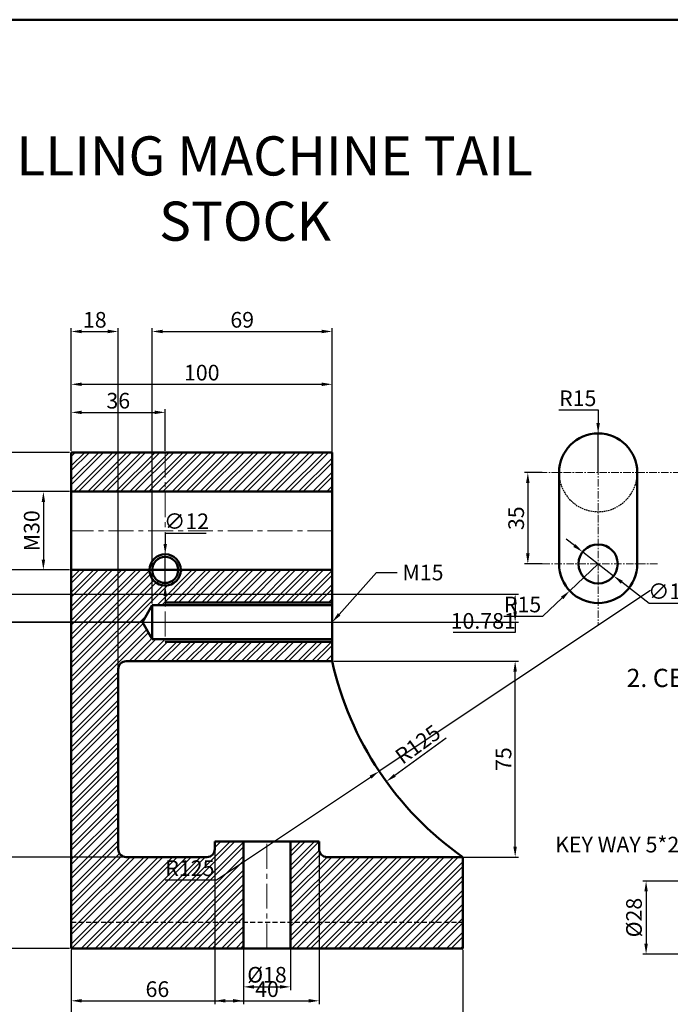
# Model space of a CAD drawing. Units: millimetres. Extents: x 177 to 1064, y 105 to 671.
# Tile 3 of 4: x 480 to 730, y 294 to 671. Entities that reach past the tile are written whole.
import ezdxf
from ezdxf import colors
from ezdxf.entities.mleader import LeaderData, LeaderLine
from ezdxf.math import Vec2, Vec3

# ---------------------------------------------------------------- set-up
doc = ezdxf.new("R2010")
doc.units = ezdxf.units.MM
doc.header["$LTSCALE"] = 0.3
doc.linetypes.add('CENTER', pattern=[50.8, 31.75, -6.35, 6.35, -6.35])
doc.linetypes.add('HIDDEN', pattern=[9.525, 6.35, -3.175])
for name, color, linetype, lineweight in [('M-CNTR', 1, 'CENTER', 18), ('M-DIMS', 2, 'Continuous', 25), ('M-HATC', 8, 'Continuous', 18), ('M-HIDN', 6, 'HIDDEN', 25), ('M-OUTL', 7, 'Continuous', 50), ('M-TEXT', 3, 'Continuous', 25)]:
    doc.layers.add(name, color=color, linetype=linetype, lineweight=lineweight)
doc.styles.get("Standard").update_dxf_attribs({"font": 'arial.ttf'})
doc.dimstyles.new('ISO-25', dxfattribs={"dimtxt": 6, "dimasz": 4, "dimexe": 1.25, "dimexo": 0.625, "dimtad": 1, "dimtoh": 1, "dimtxsty": 'Standard', "dimcen": 2.5, "dimadec": 0, "dimazin": 0, "dimtfac": 1, "dimtmove": 0, "dimatfit": 3, "dimfxl": 1, "dimarcsym": 0})

# ---------------------------------------------------------------- blocks, each defined once
blk = doc.blocks.new('*D14')
at = {"layer": 'Defpoints', "color": 0, "ltscale": 0.2, "transparency": 16777216}
for p in [(600.2, 531.47), (500.2, 505.34), (600.2, 505.34)]:
    blk.add_point(p, dxfattribs=at)
at = {"layer": 'M-DIMS', "color": 0, "lineweight": -2, "ltscale": 0.2, "transparency": 16777216}
for p, q in [((500.2, 505.97), (500.2, 532.72)), ((600.2, 505.97), (600.2, 532.72)), ((504.2, 531.47), (596.2, 531.47))]:
    blk.add_line(p, q, dxfattribs=at)
at = {"layer": 'M-DIMS', "color": 0, "ltscale": 0.2, "transparency": 16777216}
for points in [[(504.2, 532.14), (504.2, 530.81), (500.2, 531.47)], [(596.2, 532.14), (596.2, 530.81), (600.2, 531.47)]]:
    blk.add_solid(points, dxfattribs=at)
at = {"layer": 'M-DIMS', "color": 0, "ltscale": 0.2, "transparency": 16777216, "insert": (550.2, 535.16), "char_height": 6, "attachment_point": 5}
blk.add_mtext('100', dxfattribs=at)
blk = doc.blocks.new('*D15')
at = {"layer": 'Defpoints', "color": 0, "ltscale": 0.2, "transparency": 16777216}
for p in [(536.2, 520.72), (500.2, 505.34), (536.2, 505.34)]:
    blk.add_point(p, dxfattribs=at)
at = {"layer": 'M-DIMS', "color": 0, "lineweight": -2, "ltscale": 0.2, "transparency": 16777216}
for p, q in [((500.2, 505.97), (500.2, 521.97)), ((504.2, 520.72), (532.2, 520.72)), ((536.2, 505.97), (536.2, 521.97))]:
    blk.add_line(p, q, dxfattribs=at)
at = {"layer": 'M-DIMS', "color": 0, "ltscale": 0.2, "transparency": 16777216}
for points in [[(504.2, 521.38), (504.2, 520.05), (500.2, 520.72)], [(532.2, 521.38), (532.2, 520.05), (536.2, 520.72)]]:
    blk.add_solid(points, dxfattribs=at)
at = {"layer": 'M-DIMS', "color": 0, "ltscale": 0.2, "transparency": 16777216, "insert": (518.2, 524.41), "char_height": 6, "attachment_point": 5}
blk.add_mtext('36', dxfattribs=at)
blk = doc.blocks.new('*D16')
at = {"layer": 'Defpoints', "color": 0, "ltscale": 0.2, "transparency": 16777216}
for p in [(500.2, 490.34), (489.5, 460.34), (500.2, 460.34)]:
    blk.add_point(p, dxfattribs=at)
at = {"layer": 'M-DIMS', "color": 0, "lineweight": -2, "ltscale": 0.2, "transparency": 16777216}
for p, q in [((499.57, 490.34), (488.25, 490.34)), ((489.5, 486.34), (489.5, 464.34)), ((499.57, 460.34), (488.25, 460.34))]:
    blk.add_line(p, q, dxfattribs=at)
at = {"layer": 'M-DIMS', "color": 0, "ltscale": 0.2, "transparency": 16777216}
for points in [[(488.84, 486.34), (490.17, 486.34), (489.5, 490.34)], [(488.84, 464.34), (490.17, 464.34), (489.5, 460.34)]]:
    blk.add_solid(points, dxfattribs=at)
at = {"layer": 'M-DIMS', "color": 0, "ltscale": 0.2, "transparency": 16777216, "insert": (485.81, 475.34), "char_height": 6, "attachment_point": 5, "rotation": 90}
blk.add_mtext('M30', dxfattribs=at)
blk = doc.blocks.new('*D17')
at = {"layer": 'Defpoints', "color": 0, "ltscale": 0.2, "transparency": 16777216}
for p in [(500.2, 315.34), (650.2, 315.34), (650.2, 279.36)]:
    blk.add_point(p, dxfattribs=at)
at = {"layer": 'M-DIMS', "color": 0, "lineweight": -2, "ltscale": 0.2, "transparency": 16777216}
for p, q in [((500.2, 314.72), (500.2, 278.11)), ((650.2, 314.72), (650.2, 278.11)), ((504.2, 279.36), (646.2, 279.36))]:
    blk.add_line(p, q, dxfattribs=at)
at = {"layer": 'M-DIMS', "color": 0, "ltscale": 0.2, "transparency": 16777216}
for points in [[(504.2, 280.03), (504.2, 278.7), (500.2, 279.36)], [(646.2, 280.03), (646.2, 278.7), (650.2, 279.36)]]:
    blk.add_solid(points, dxfattribs=at)
at = {"layer": 'M-DIMS', "color": 0, "ltscale": 0.2, "transparency": 16777216, "insert": (575.2, 283.05), "char_height": 6, "attachment_point": 5}
blk.add_mtext('150', dxfattribs=at)
blk = doc.blocks.new('*D18')
at = {"layer": 'Defpoints', "color": 0, "ltscale": 0.2, "transparency": 16777216}
for p in [(566.2, 315.34), (584.2, 315.34), (584.2, 300.59)]:
    blk.add_point(p, dxfattribs=at)
at = {"layer": 'M-DIMS', "color": 0, "lineweight": -2, "ltscale": 0.2, "transparency": 16777216}
for p, q in [((566.2, 314.72), (566.2, 299.34)), ((584.2, 314.72), (584.2, 299.34)), ((570.2, 300.59), (580.2, 300.59))]:
    blk.add_line(p, q, dxfattribs=at)
at = {"layer": 'M-DIMS', "color": 0, "ltscale": 0.2, "transparency": 16777216}
for points in [[(570.2, 301.25), (570.2, 299.92), (566.2, 300.59)], [(580.2, 301.25), (580.2, 299.92), (584.2, 300.59)]]:
    blk.add_solid(points, dxfattribs=at)
at = {"layer": 'M-DIMS', "color": 0, "ltscale": 0.2, "transparency": 16777216, "insert": (575.2, 304.44), "char_height": 6, "attachment_point": 5}
blk.add_mtext('%%C18', dxfattribs=at)
blk = doc.blocks.new('*D19')
at = {"layer": 'Defpoints', "color": 0, "ltscale": 0.2, "transparency": 16777216}
for p in [(722.21, 452.52), (620.92, 379.27)]:
    blk.add_point(p, dxfattribs=at)
at = {"layer": 'M-DIMS', "color": 0, "lineweight": -2, "ltscale": 0.2, "transparency": 16777216}
blk.add_line((643.85, 395.85), (624.16, 381.61), dxfattribs=at)
at = {"layer": 'M-DIMS', "color": 0, "ltscale": 0.2, "transparency": 16777216}
blk.add_solid([(623.77, 382.15), (624.55, 381.07), (620.92, 379.27)], dxfattribs=at)
at = {"layer": 'M-DIMS', "color": 0, "ltscale": 0.2, "transparency": 16777216, "insert": (633.46, 392.89), "char_height": 6, "attachment_point": 5, "rotation": 35.8741}
blk.add_mtext('R125', dxfattribs=at)
blk = doc.blocks.new('*D23')
at = {"layer": 'Defpoints', "color": 0, "ltscale": 0.3, "transparency": 16777216}
for p in [(681.26, 497.65), (675.16, 462.65), (681.26, 462.65)]:
    blk.add_point(p, dxfattribs=at)
at = {"layer": 'M-DIMS', "color": 0, "lineweight": -2, "ltscale": 0.3, "transparency": 16777216}
for p, q in [((680.64, 497.65), (673.91, 497.65)), ((675.16, 493.65), (675.16, 466.65)), ((680.64, 462.65), (673.91, 462.65))]:
    blk.add_line(p, q, dxfattribs=at)
at = {"layer": 'M-DIMS', "color": 0, "ltscale": 0.3, "transparency": 16777216}
for points in [[(674.49, 493.65), (675.83, 493.65), (675.16, 497.65)], [(674.49, 466.65), (675.83, 466.65), (675.16, 462.65)]]:
    blk.add_solid(points, dxfattribs=at)
at = {"layer": 'M-DIMS', "color": 0, "ltscale": 0.3, "transparency": 16777216, "insert": (671.47, 480.15), "char_height": 6, "attachment_point": 5, "rotation": 90}
blk.add_mtext('35', dxfattribs=at)
blk = doc.blocks.new('*D24')
at = {"layer": 'Defpoints', "color": 0, "ltscale": 0.3, "transparency": 16777216}
for p in [(702.11, 462.65), (691.21, 452.34)]:
    blk.add_point(p, dxfattribs=at)
at = {"layer": 'M-DIMS', "color": 0, "lineweight": -2, "ltscale": 0.3, "transparency": 16777216}
for p, q in [((702.11, 462.65), (691.21, 452.34)), ((680.95, 442.64), (688.31, 449.6)), ((665.94, 442.64), (680.95, 442.64))]:
    blk.add_line(p, q, dxfattribs=at)
at = {"layer": 'M-DIMS', "color": 0, "ltscale": 0.3, "transparency": 16777216}
blk.add_solid([(687.85, 450.08), (688.77, 449.11), (691.21, 452.34)], dxfattribs=at)
at = {"layer": 'M-DIMS', "color": 0, "ltscale": 0.3, "transparency": 16777216, "insert": (673.13, 446.33), "char_height": 6, "attachment_point": 5}
blk.add_mtext('R15', dxfattribs=at)
blk = doc.blocks.new('*D25')
at = {"layer": 'Defpoints', "color": 0, "ltscale": 0.3, "transparency": 16777216}
for p in [(696.18, 467.24), (708.04, 458.06)]:
    blk.add_point(p, dxfattribs=at)
at = {"layer": 'M-DIMS', "color": 0, "lineweight": -2, "ltscale": 0.3, "transparency": 16777216}
for p, q in [((693.02, 469.69), (689.85, 472.14)), ((696.18, 467.24), (708.04, 458.06)), ((721.67, 447.51), (711.2, 455.61)), ((737.46, 447.51), (721.67, 447.51))]:
    blk.add_line(p, q, dxfattribs=at)
at = {"layer": 'M-DIMS', "color": 0, "ltscale": 0.3, "transparency": 16777216}
for points in [[(693.43, 470.22), (692.61, 469.16), (696.18, 467.24)], [(711.61, 456.14), (710.8, 455.08), (708.04, 458.06)]]:
    blk.add_solid(points, dxfattribs=at)
at = {"layer": 'M-DIMS', "color": 0, "ltscale": 0.3, "transparency": 16777216, "insert": (729.88, 451.37), "char_height": 6, "attachment_point": 5}
blk.add_mtext('∅15', dxfattribs=at)
blk = doc.blocks.new('*D29')
at = {"layer": 'Defpoints', "color": 0, "ltscale": 0.3, "transparency": 16777216}
for p in [(748.87, 341.13), (720.48, 313.13), (748.87, 313.13)]:
    blk.add_point(p, dxfattribs=at)
at = {"layer": 'M-DIMS', "color": 0, "lineweight": -2, "ltscale": 0.3, "transparency": 16777216}
for p, q in [((748.24, 341.13), (719.23, 341.13)), ((720.48, 337.13), (720.48, 317.13)), ((748.24, 313.13), (719.23, 313.13))]:
    blk.add_line(p, q, dxfattribs=at)
at = {"layer": 'M-DIMS', "color": 0, "ltscale": 0.3, "transparency": 16777216}
for points in [[(719.81, 337.13), (721.14, 337.13), (720.48, 341.13)], [(719.81, 317.13), (721.14, 317.13), (720.48, 313.13)]]:
    blk.add_solid(points, dxfattribs=at)
at = {"layer": 'M-DIMS', "color": 0, "ltscale": 0.3, "transparency": 16777216, "insert": (716.62, 327.13), "char_height": 6, "attachment_point": 5, "rotation": 90}
blk.add_mtext('%%C28', dxfattribs=at)
blk = doc.blocks.new('*D51')
at = {"layer": 'Defpoints', "color": 0, "ltscale": 0.3, "transparency": 16777216}
for p in [(409.04, 451.12), (377.04, 440.34), (670.3, 440.34)]:
    blk.add_point(p, dxfattribs=at)
at = {"layer": 'M-DIMS', "color": 0, "lineweight": -2, "ltscale": 0.3, "transparency": 16777216}
for p, q in [((409.67, 451.12), (671.55, 451.12)), ((670.3, 447.12), (670.3, 444.34)), ((377.67, 440.34), (671.55, 440.34)), ((670.3, 440.34), (670.3, 436.34)), ((670.3, 436.34), (646.49, 436.34))]:
    blk.add_line(p, q, dxfattribs=at)
at = {"layer": 'M-DIMS', "color": 0, "ltscale": 0.3, "transparency": 16777216}
for points in [[(669.63, 447.12), (670.96, 447.12), (670.3, 451.12)], [(669.63, 444.34), (670.96, 444.34), (670.3, 440.34)]]:
    blk.add_solid(points, dxfattribs=at)
at = {"layer": 'M-DIMS', "color": 0, "ltscale": 0.3, "transparency": 16777216, "insert": (658.08, 440.03), "char_height": 6, "attachment_point": 5}
blk.add_mtext('10.781', dxfattribs=at)
blk = doc.blocks.new('*D53')
at = {"layer": 'Defpoints', "color": 0, "ltscale": 0.3, "transparency": 16777216}
for p in [(518.2, 551.72), (500.2, 505.34), (518.2, 422.34)]:
    blk.add_point(p, dxfattribs=at)
at = {"layer": 'M-DIMS', "color": 0, "lineweight": -2, "ltscale": 0.3, "transparency": 16777216}
for p, q in [((500.2, 505.97), (500.2, 552.97)), ((504.2, 551.72), (514.2, 551.72)), ((518.2, 422.97), (518.2, 552.97))]:
    blk.add_line(p, q, dxfattribs=at)
at = {"layer": 'M-DIMS', "color": 0, "ltscale": 0.3, "transparency": 16777216}
for points in [[(504.2, 552.39), (504.2, 551.05), (500.2, 551.72)], [(514.2, 552.39), (514.2, 551.05), (518.2, 551.72)]]:
    blk.add_solid(points, dxfattribs=at)
at = {"layer": 'M-DIMS', "color": 0, "ltscale": 0.3, "transparency": 16777216, "insert": (509.2, 555.41), "char_height": 6, "attachment_point": 5}
blk.add_mtext('18', dxfattribs=at)
blk = doc.blocks.new('*D54')
at = {"layer": 'Defpoints', "color": 0, "ltscale": 0.3, "transparency": 16777216}
for p in [(500.2, 505.34), (265.25, 490.34), (500.2, 490.34)]:
    blk.add_point(p, dxfattribs=at)
at = {"layer": 'M-DIMS', "color": 0, "lineweight": -2, "ltscale": 0.3, "transparency": 16777216}
for p, q in [((499.57, 505.34), (264, 505.34)), ((265.25, 501.34), (265.25, 494.34)), ((499.57, 490.34), (264, 490.34))]:
    blk.add_line(p, q, dxfattribs=at)
at = {"layer": 'M-DIMS', "color": 0, "ltscale": 0.3, "transparency": 16777216}
for points in [[(264.58, 501.34), (265.92, 501.34), (265.25, 505.34)], [(264.58, 494.34), (265.92, 494.34), (265.25, 490.34)]]:
    blk.add_solid(points, dxfattribs=at)
at = {"layer": 'M-DIMS', "color": 0, "ltscale": 0.3, "transparency": 16777216, "insert": (261.56, 497.84), "char_height": 6, "attachment_point": 5, "rotation": 90}
blk.add_mtext('15', dxfattribs=at)
blk = doc.blocks.new('*D55')
at = {"layer": 'Defpoints', "color": 0, "ltscale": 0.3, "transparency": 16777216}
for p in [(265.25, 460.34), (500.2, 460.34), (527.44, 440.34)]:
    blk.add_point(p, dxfattribs=at)
at = {"layer": 'M-DIMS', "color": 0, "lineweight": -2, "ltscale": 0.3, "transparency": 16777216}
for p, q in [((499.57, 460.34), (264, 460.34)), ((265.25, 444.34), (265.25, 456.34)), ((526.82, 440.34), (264, 440.34))]:
    blk.add_line(p, q, dxfattribs=at)
at = {"layer": 'M-DIMS', "color": 0, "ltscale": 0.3, "transparency": 16777216}
for points in [[(264.58, 456.34), (265.92, 456.34), (265.25, 460.34)], [(264.58, 444.34), (265.92, 444.34), (265.25, 440.34)]]:
    blk.add_solid(points, dxfattribs=at)
at = {"layer": 'M-DIMS', "color": 0, "ltscale": 0.3, "transparency": 16777216, "insert": (261.56, 450.34), "char_height": 6, "attachment_point": 5, "rotation": 90}
blk.add_mtext('20', dxfattribs=at)
blk = doc.blocks.new('*D56')
at = {"layer": 'Defpoints', "color": 0, "ltscale": 0.3, "transparency": 16777216}
for p in [(600.2, 425.34), (670.3, 425.34), (650.2, 350.34)]:
    blk.add_point(p, dxfattribs=at)
at = {"layer": 'M-DIMS', "color": 0, "lineweight": -2, "ltscale": 0.3, "transparency": 16777216}
for p, q in [((600.82, 425.34), (671.55, 425.34)), ((670.3, 354.34), (670.3, 421.34)), ((650.82, 350.34), (671.55, 350.34))]:
    blk.add_line(p, q, dxfattribs=at)
at = {"layer": 'M-DIMS', "color": 0, "ltscale": 0.3, "transparency": 16777216}
for points in [[(669.63, 421.34), (670.96, 421.34), (670.3, 425.34)], [(669.63, 354.34), (670.96, 354.34), (670.3, 350.34)]]:
    blk.add_solid(points, dxfattribs=at)
at = {"layer": 'M-DIMS', "color": 0, "ltscale": 0.3, "transparency": 16777216, "insert": (666.62, 387.84), "char_height": 6, "attachment_point": 5, "rotation": 90}
blk.add_mtext('75', dxfattribs=at)
blk = doc.blocks.new('*D57')
at = {"layer": 'Defpoints', "color": 0, "ltscale": 0.3, "transparency": 16777216}
for p in [(521.2, 350.34), (265.25, 315.34), (500.2, 315.34)]:
    blk.add_point(p, dxfattribs=at)
at = {"layer": 'M-DIMS', "color": 0, "lineweight": -2, "ltscale": 0.3, "transparency": 16777216}
for p, q in [((520.57, 350.34), (264, 350.34)), ((265.25, 346.34), (265.25, 319.34)), ((499.57, 315.34), (264, 315.34))]:
    blk.add_line(p, q, dxfattribs=at)
at = {"layer": 'M-DIMS', "color": 0, "ltscale": 0.3, "transparency": 16777216}
for points in [[(264.58, 346.34), (265.92, 346.34), (265.25, 350.34)], [(264.58, 319.34), (265.92, 319.34), (265.25, 315.34)]]:
    blk.add_solid(points, dxfattribs=at)
at = {"layer": 'M-DIMS', "color": 0, "ltscale": 0.3, "transparency": 16777216, "insert": (261.56, 332.84), "char_height": 6, "attachment_point": 5, "rotation": 90}
blk.add_mtext('35', dxfattribs=at)
blk = doc.blocks.new('*D58')
at = {"layer": 'Defpoints', "color": 0, "ltscale": 0.3, "transparency": 16777216}
for p in [(500.2, 315.34), (566.2, 315.34), (566.2, 295.24)]:
    blk.add_point(p, dxfattribs=at)
at = {"layer": 'M-DIMS', "color": 0, "lineweight": -2, "ltscale": 0.3, "transparency": 16777216}
for p, q in [((500.2, 314.72), (500.2, 293.99)), ((566.2, 314.72), (566.2, 293.99)), ((504.2, 295.24), (562.2, 295.24))]:
    blk.add_line(p, q, dxfattribs=at)
at = {"layer": 'M-DIMS', "color": 0, "ltscale": 0.3, "transparency": 16777216}
for points in [[(504.2, 295.91), (504.2, 294.58), (500.2, 295.24)], [(562.2, 295.91), (562.2, 294.58), (566.2, 295.24)]]:
    blk.add_solid(points, dxfattribs=at)
at = {"layer": 'M-DIMS', "color": 0, "ltscale": 0.3, "transparency": 16777216, "insert": (533.2, 298.93), "char_height": 6, "attachment_point": 5}
blk.add_mtext('66', dxfattribs=at)
blk = doc.blocks.new('*D59')
at = {"layer": 'Defpoints', "color": 0, "ltscale": 0.3, "transparency": 16777216}
for p in [(600.2, 551.72), (531.2, 446.84), (600.2, 446.84)]:
    blk.add_point(p, dxfattribs=at)
at = {"layer": 'M-DIMS', "color": 0, "lineweight": -2, "ltscale": 0.3, "transparency": 16777216}
for p, q in [((531.2, 447.47), (531.2, 552.97)), ((535.2, 551.72), (596.2, 551.72)), ((600.2, 447.47), (600.2, 552.97))]:
    blk.add_line(p, q, dxfattribs=at)
at = {"layer": 'M-DIMS', "color": 0, "ltscale": 0.3, "transparency": 16777216}
for points in [[(535.2, 552.39), (535.2, 551.05), (531.2, 551.72)], [(596.2, 552.39), (596.2, 551.05), (600.2, 551.72)]]:
    blk.add_solid(points, dxfattribs=at)
at = {"layer": 'M-DIMS', "color": 0, "ltscale": 0.3, "transparency": 16777216, "insert": (565.7, 555.41), "char_height": 6, "attachment_point": 5}
blk.add_mtext('69', dxfattribs=at)
blk = doc.blocks.new('*D60')
at = {"layer": 'Defpoints', "color": 0, "ltscale": 0.3, "transparency": 16777216}
for p in [(555.2, 356.34), (595.2, 356.34), (595.2, 295.24)]:
    blk.add_point(p, dxfattribs=at)
at = {"layer": 'M-DIMS', "color": 0, "lineweight": -2, "ltscale": 0.3, "transparency": 16777216}
for p, q in [((555.2, 355.72), (555.2, 293.99)), ((595.2, 355.72), (595.2, 293.99)), ((559.2, 295.24), (591.2, 295.24))]:
    blk.add_line(p, q, dxfattribs=at)
at = {"layer": 'M-DIMS', "color": 0, "ltscale": 0.3, "transparency": 16777216}
for points in [[(559.2, 295.91), (559.2, 294.58), (555.2, 295.24)], [(591.2, 295.91), (591.2, 294.58), (595.2, 295.24)]]:
    blk.add_solid(points, dxfattribs=at)
at = {"layer": 'M-DIMS', "color": 0, "ltscale": 0.3, "transparency": 16777216, "insert": (575.2, 298.93), "char_height": 6, "attachment_point": 5}
blk.add_mtext('40', dxfattribs=at)
blk = doc.blocks.new('*D70')
at = {"layer": 'Defpoints', "color": 0, "ltscale": 0.3, "transparency": 16777216}
for p in [(722.21, 452.52), (618.2, 383.18)]:
    blk.add_point(p, dxfattribs=at)
at = {"layer": 'M-DIMS', "color": 0, "lineweight": -2, "ltscale": 0.3, "transparency": 16777216}
for p, q in [((722.21, 452.52), (618.2, 383.18)), ((555.8, 341.58), (614.87, 380.96)), ((536.13, 341.58), (555.8, 341.58))]:
    blk.add_line(p, q, dxfattribs=at)
at = {"layer": 'M-DIMS', "color": 0, "ltscale": 0.3, "transparency": 16777216}
blk.add_solid([(614.5, 381.51), (615.24, 380.41), (618.2, 383.18)], dxfattribs=at)
at = {"layer": 'M-DIMS', "color": 0, "ltscale": 0.3, "transparency": 16777216, "insert": (545.65, 345.27), "char_height": 6, "attachment_point": 5}
blk.add_mtext('R125', dxfattribs=at)
blk = doc.blocks.new('*D71')
at = {"layer": 'Defpoints', "color": 0, "ltscale": 0.3, "transparency": 16777216}
for p in [(536.2, 466.34), (536.19, 454.34)]:
    blk.add_point(p, dxfattribs=at)
at = {"layer": 'M-DIMS', "color": 0, "lineweight": -2, "ltscale": 0.3, "transparency": 16777216}
for p, q in [((551.89, 474.34), (536.2, 474.34)), ((536.2, 474.34), (536.2, 470.34)), ((536.19, 454.34), (536.2, 466.34)), ((536.19, 450.34), (536.19, 446.34))]:
    blk.add_line(p, q, dxfattribs=at)
at = {"layer": 'M-DIMS', "color": 0, "ltscale": 0.3, "transparency": 16777216}
for points in [[(535.54, 470.34), (536.87, 470.34), (536.2, 466.34)], [(535.52, 450.34), (536.86, 450.34), (536.19, 454.34)]]:
    blk.add_solid(points, dxfattribs=at)
at = {"layer": 'M-DIMS', "color": 0, "ltscale": 0.3, "transparency": 16777216, "insert": (544.36, 478.2), "char_height": 6, "attachment_point": 5}
blk.add_mtext('∅12', dxfattribs=at)
blk = doc.blocks.new('*D72')
at = {"layer": 'Defpoints', "color": 0, "ltscale": 0.3, "transparency": 16777216}
for p in [(702.11, 512.65), (702.11, 497.65)]:
    blk.add_point(p, dxfattribs=at)
at = {"layer": 'M-DIMS', "color": 0, "lineweight": -2, "ltscale": 0.3, "transparency": 16777216}
for p, q in [((687.1, 521.65), (702.11, 521.65)), ((702.11, 521.65), (702.11, 516.65)), ((702.11, 497.65), (702.11, 512.65))]:
    blk.add_line(p, q, dxfattribs=at)
at = {"layer": 'M-DIMS', "color": 0, "ltscale": 0.3, "transparency": 16777216}
blk.add_solid([(702.78, 516.65), (701.44, 516.65), (702.11, 512.65)], dxfattribs=at)
at = {"layer": 'M-DIMS', "color": 0, "ltscale": 0.3, "transparency": 16777216, "insert": (694.29, 525.34), "char_height": 6, "attachment_point": 5}
blk.add_mtext('R15', dxfattribs=at)

msp = doc.modelspace()

# ---------------------------------------------------------------- hatches: boundary and pattern name
at = {"layer": 'M-HATC', "ltscale": 0.2}
h = msp.add_hatch(dxfattribs=at)
h.set_pattern_fill('ANSI32', color=256, scale=0.4)
h.paths.add_polyline_path([(600.1968, 505.3423), (536.1968, 505.3423), (536.1968, 490.3423), (600.1968, 490.3423)])
h.paths.add_polyline_path([(536.1968, 505.3423), (500.1968, 505.3423), (500.1968, 490.3423), (536.1968, 490.3423)])
h = msp.add_hatch(dxfattribs=at)
h.set_pattern_fill('ANSI32', color=256, scale=0.4)
h.paths.add_polyline_path([(531.1968, 446.8423), (536.1968, 446.8423), (536.1968, 454.3423, -0.41421356), (530.1968, 460.3423), (500.1968, 460.3423), (500.1968, 325.3423), (566.1968, 325.3423), (566.1968, 356.3423), (555.1968, 356.3423), (555.1968, 353.3423, -0.41421356), (552.1968, 350.3423), (521.1968, 350.3423, -0.41421356), (518.1968, 353.3423), (518.1968, 422.3423, -0.41421356), (521.1968, 425.3423), (600.1968, 425.3423), (600.1968, 432.8423), (536.1968, 432.8423), (536.1968, 433.8423), (531.1968, 433.8423), (527.444, 440.3423)])
h.paths.add_polyline_path([(600.1968, 460.3423), (542.1968, 460.3423, -0.41421356), (536.1968, 454.3423), (536.1968, 447.8423), (600.1968, 447.8423)], flags=17)
h.paths.add_polyline_path([(650.1968, 350.3423), (598.1968, 350.3423, -0.41421356), (595.1968, 353.3423), (595.1968, 356.3423), (584.1968, 356.3423), (584.1968, 325.3423), (650.1968, 325.3423)])
h.paths.add_polyline_path([(566.1968, 325.3423), (500.1968, 325.3423), (500.1968, 315.3423), (566.1968, 315.3423)])
h.paths.add_polyline_path([(650.1968, 325.3423), (584.1968, 325.3423), (584.1968, 315.3423), (650.1968, 315.3423)])

# ---------------------------------------------------------------- linework, layer by layer
at = {"layer": 'M-CNTR', "ltscale": 0.3}
for p, q in [((702.1114, 517.9895), (702.1114, 439.2537)), ((675.1472, 497.6506), (717.1114, 497.6506)), ((717.1114, 497.6506), (953.625, 497.6506)), ((680.7852, 462.6506), (724.8556, 462.6506))]:
    msp.add_line(p, q, dxfattribs=at)
at = {"layer": 'M-CNTR'}
for p, q in [((536.1968, 505.3423), (536.1968, 432.8423)), ((600.1968, 475.3423), (500.1968, 475.3423)), ((600.1968, 440.3423), (527.444, 440.3423)), ((575.1968, 315.3423), (575.1968, 356.3423))]:
    msp.add_line(p, q, dxfattribs=at)
at = {"layer": 'M-HIDN'}
msp.add_line((500.1968, 325.3423), (650.1968, 325.3423), dxfattribs=at)
at = {"layer": 'M-HIDN', "ltscale": 0.3}
msp.add_arc((702.1114, 497.6506), 15, 180, 0, dxfattribs=at)
at = {"layer": 'M-OUTL'}
for p, q in [((500.1968, 505.3423), (600.1968, 505.3423)), ((500.1968, 505.3423), (500.1968, 315.3423)), ((600.1968, 505.3423), (600.1968, 440.3423)), ((600.1968, 490.3423), (500.1968, 490.3423)), ((600.1968, 460.3423), (500.1968, 460.3423)), ((600.1968, 425.3423), (600.1968, 440.3423)), ((521.1968, 425.3423), (600.1968, 425.3423)), ((518.1968, 422.3423), (518.1968, 353.3423)), ((555.1968, 353.3423), (555.1968, 356.3423)), ((555.1968, 356.3423), (595.1968, 356.3423)), ((566.1968, 315.3423), (566.1968, 356.3423)), ((584.1968, 315.3423), (584.1968, 356.3423)), ((595.1968, 353.3423), (595.1968, 356.3423)), ((552.1968, 350.3423), (521.1968, 350.3423)), ((650.1968, 350.3423), (598.1968, 350.3423)), ((650.1968, 315.3423), (650.1968, 350.3423)), ((500.1968, 315.3423), (650.1968, 315.3423))]:
    msp.add_line(p, q, dxfattribs=at)
at = {"layer": 'M-OUTL', "ltscale": 0.3}
for p, q in [((687.1114, 497.6506), (687.1114, 462.6506)), ((717.1114, 497.6506), (717.1114, 462.6506))]:
    msp.add_line(p, q, dxfattribs=at)
at = {"layer": 'M-OUTL', "ltscale": 0.2}
for p, q in [((531.1968, 446.8423), (527.444, 440.3423)), ((536.1968, 446.8423), (531.1968, 446.8423)), ((531.1968, 446.8423), (531.1968, 433.8423)), ((536.1968, 447.8423), (600.1968, 447.8423)), ((536.1968, 446.8423), (600.1968, 446.8423)), ((531.1968, 433.8423), (527.444, 440.3423)), ((531.1968, 433.8423), (536.1968, 433.8423)), ((536.1968, 433.8423), (600.1968, 433.8423)), ((536.1968, 432.8423), (600.1968, 432.8423))]:
    msp.add_line(p, q, dxfattribs=at)
at = {"layer": 'M-OUTL', "ltscale": 0.3}
msp.add_lwpolyline([(176.7558, 671.1865), (1063.6064, 671.1865), (1063.6064, 105.1095), (176.7558, 105.1095)], close=True, dxfattribs=at)
msp.add_circle((702.1114, 462.6506), 7.5, dxfattribs=at)
at = {"layer": 'M-OUTL'}
for radius in [6, 5]:
    msp.add_circle((536.1968, 460.3423), radius, dxfattribs=at)
at = {"layer": 'M-OUTL', "ltscale": 0.3}
for centre, start, end in [((702.1114, 497.6506), 0, 180), ((702.1114, 462.6506), 180, 0)]:
    msp.add_arc(centre, 15, start, end, dxfattribs=at)
at = {"layer": 'M-OUTL'}
for centre, start, end in [((521.1968, 422.3423), 90, 180), ((521.1968, 353.3423), 180, 270), ((552.1968, 353.3423), 270, 0), ((598.1968, 353.3423), 180, 270)]:
    msp.add_arc(centre, 3, start, end, dxfattribs=at)
at = {"layer": 'M-OUTL', "ltscale": 0.2}
msp.add_arc((722.2074, 452.5161), 125, 192.555775, 234.82436, dxfattribs=at)

# ---------------------------------------------------------------- texts
at = {"layer": 'M-TEXT', "ltscale": 0.3, "attachment_point": 1}
for s, width, insert, char_height in [('\\pxqc;MILLING MACHINE TAIL STOCK', 257.833122, (437.8929, 626.4883), 15), ('\\pxqc;2. CENTRE (CASE HARDENED ALLOY STEEL) NO.1', 275.896457, (682.4091, 422.4621), 7)]:
    msp.add_mtext_dynamic_manual_height_columns(s, width=width, gutter_width=12.5, heights=[0], dxfattribs=dict(at, insert=insert, char_height=char_height))

# ---------------------------------------------------------------- dimensions: what is measured, and where the dimension line sits
at = {"layer": 'M-DIMS', "ltscale": 0.3}
for base, p1, p2, picture, middle in [((518.1968, 551.7184), (500.1968, 505.3423), (518.1968, 422.3423), '*D53', (509.1968, 555.4068)), ((600.1968, 551.7184), (531.1968, 446.8423), (600.1968, 446.8423), '*D59', (565.6968, 555.4068)), ((595.1968, 295.2423), (555.1968, 356.3423), (595.1968, 356.3423), '*D60', (575.1968, 298.9308)), ((566.1968, 295.2423), (500.1968, 315.3423), (566.1968, 315.3423), '*D58', (533.1968, 298.9308))]:
    dim = msp.add_linear_dim(base=base, p1=p1, p2=p2, dimstyle='ISO-25', override={"dimdec": 0, "dimlfac": 1, "dimrnd": 0, "dimzin": 0, "dimdsep": 46, "dimlunit": 2}, dxfattribs=at)
    dim.commit()
    dim.dimension.update_dxf_attribs({"geometry": picture, "text_midpoint": middle})
at = {"layer": 'M-DIMS', "ltscale": 0.2}
for base, p1, p2, picture, middle in [((600.1968, 531.4739), (500.1968, 505.3423), (600.1968, 505.3423), '*D14', (550.1968, 535.1623)), ((536.1968, 520.7167), (500.1968, 505.3423), (536.1968, 505.3423), '*D15', (518.1968, 524.4072)), ((650.1968, 279.3639), (500.1968, 315.3423), (650.1968, 315.3423), '*D17', (575.1968, 283.0523))]:
    dim = msp.add_linear_dim(base=base, p1=p1, p2=p2, dimstyle='ISO-25', override={"dimclrd": 0, "dimclre": 0, "dimclrt": 0}, dxfattribs=at)
    dim.commit()
    dim.dimension.update_dxf_attribs({"geometry": picture, "text_midpoint": middle})
at = {"layer": 'M-DIMS', "ltscale": 0.3}
for center, mpoint, picture, middle in [((702.1114, 497.6506), (702.111, 512.6506), '*D72', (694.2948, 521.6506)), ((722.2074, 452.5161), (618.2009, 383.1789), '*D70', (545.6501, 341.5766))]:
    dim = msp.add_radius_dim(center=center, mpoint=mpoint, dimstyle='ISO-25', override={"dimdec": 0, "dimlfac": 1, "dimrnd": 0, "dimzin": 0, "dimdsep": 46, "dimlunit": 2}, dxfattribs=at)
    dim.commit()
    dim.dimension.update_dxf_attribs({"geometry": picture, "text_midpoint": middle, "dimtype": 164})
for base, p1, p2, override, picture, middle in [((265.2513, 490.3423), (500.1968, 505.3423), (500.1968, 490.3423), {"dimdec": 0, "dimlfac": 1, "dimrnd": 0, "dimzin": 0, "dimdsep": 46, "dimlunit": 2}, '*D54', (261.5629, 497.8423)), ((675.159, 462.6506), (681.2617, 497.6506), (681.2617, 462.6506), {"dimclrd": 0, "dimclre": 0, "dimclrt": 0}, '*D23', (671.4685, 480.1506)), ((265.2513, 460.3423), (527.444, 440.3423), (500.1968, 460.3423), {"dimdec": 0, "dimlfac": 1, "dimrnd": 0, "dimzin": 0, "dimdsep": 46, "dimlunit": 2}, '*D55', (261.5629, 450.3423)), ((670.2968, 440.3423), (409.0432, 451.1235), (377.0432, 440.3423), {"dimdec": 3, "dimlfac": 1, "dimrnd": 0, "dimzin": 0, "dimdsep": 46, "dimlunit": 2}, '*D51', (658.079, 440.0308)), ((670.2968, 425.3423), (650.1968, 350.3423), (600.1968, 425.3423), {"dimdec": 0, "dimlfac": 1, "dimrnd": 0, "dimzin": 0, "dimdsep": 46, "dimlunit": 2}, '*D56', (666.6206, 387.8423)), ((265.2513, 315.3423), (521.1968, 350.3423), (500.1968, 315.3423), {"dimdec": 0, "dimlfac": 1, "dimrnd": 0, "dimzin": 0, "dimdsep": 46, "dimlunit": 2}, '*D57', (261.5608, 332.8423))]:
    dim = msp.add_linear_dim(base=base, p1=p1, p2=p2, angle=90, dimstyle='ISO-25', override=override, dxfattribs=at)
    dim.commit()
    dim.dimension.update_dxf_attribs({"geometry": picture, "text_midpoint": middle})
at = {"layer": 'M-DIMS', "ltscale": 0.2}
dim = msp.add_linear_dim(base=(489.5043, 460.3423), p1=(500.1968, 490.3423), p2=(500.1968, 460.3423), angle=90, text='M<>', dimstyle='ISO-25', override={"dimclrd": 0, "dimclre": 0, "dimclrt": 0}, dxfattribs=at)
dim.commit()
dim.dimension.update_dxf_attribs({"geometry": '*D16', "text_midpoint": (485.8138, 475.3423)})
at = {"layer": 'M-DIMS', "ltscale": 0.3}
for p1, p2, override, picture, middle in [((536.1936, 454.3423), (536.2, 466.3423), {"dimdec": 0, "dimlfac": 1, "dimrnd": 0, "dimzin": 0, "dimdsep": 46, "dimlunit": 2}, '*D71', (544.36, 474.3423)), ((696.1809, 467.2417), (708.042, 458.0594), {"dimclrd": 0, "dimclre": 0, "dimclrt": 0}, '*D25', (729.8751, 447.5122))]:
    dim = msp.add_diameter_dim_2p(p1=p1, p2=p2, dimstyle='ISO-25', override=override, dxfattribs=at)
    dim.commit()
    dim.dimension.update_dxf_attribs({"geometry": picture, "text_midpoint": middle, "dimtype": 163})
dim = msp.add_radius_dim(center=(702.1114, 462.6506), mpoint=(691.2134, 452.3436), dimstyle='ISO-25', override={"dimclrd": 0, "dimclre": 0, "dimclrt": 0}, dxfattribs=at)
dim.commit()
dim.dimension.update_dxf_attribs({"geometry": '*D24', "text_midpoint": (673.1338, 446.325)})
at = {"layer": 'M-DIMS', "ltscale": 0.2}
dim = msp.add_radius_dim(center=(722.2074, 452.5161), mpoint=(620.9191, 379.2653), dimstyle='ISO-25', override={"dimclrd": 0, "dimclre": 0, "dimclrt": 0}, dxfattribs=at)
dim.commit()
dim.dimension.update_dxf_attribs({"geometry": '*D19', "text_midpoint": (635.6236, 389.8994), "dimtype": 164})
at = {"layer": 'M-DIMS', "ltscale": 0.3}
dim = msp.add_linear_dim(base=(720.4777, 313.1319), p1=(748.8685, 341.1319), p2=(748.8685, 313.1319), angle=90, text='%%C<>', dimstyle='ISO-25', override={"dimclrd": 0, "dimclre": 0, "dimclrt": 0}, dxfattribs=at)
dim.commit()
dim.dimension.update_dxf_attribs({"geometry": '*D29', "text_midpoint": (716.6214, 327.1319)})
at = {"layer": 'M-DIMS', "ltscale": 0.2}
dim = msp.add_linear_dim(base=(584.1968, 300.5871), p1=(566.1968, 315.3423), p2=(584.1968, 315.3423), text='%%C<>', dimstyle='ISO-25', override={"dimclrd": 0, "dimclre": 0, "dimclrt": 0}, dxfattribs=at)
dim.commit()
dim.dimension.update_dxf_attribs({"geometry": '*D18', "text_midpoint": (575.1968, 304.4433)})

# ---------------------------------------------------------------- leaders
ml = msp.add_multileader_mtext('Standard', dxfattribs=at)
ml.set_content('M15', color=256)
ml.set_leader_properties()
ml.build(insert=Vec2(0, 0))
ctx = ml.context
ctx.base_point, ctx.char_height, ctx.plane_origin = Vec3(625.1199, 459.3104), 6, Vec3(600.1968, 440.3423)
notes = []
notes.append((ctx, [(0, (1, 1, 0), (617.1199, 459.3104), (1, 0), 8, [(0, [(600.1968, 440.3423)], 0, [])])]))
ctx.mtext.insert, ctx.mtext.flow_direction = Vec3(627.1199, 462.3616), 5
at = {"layer": 'M-DIMS', "ltscale": 0.3}
ml = msp.add_multileader_mtext('Standard', dxfattribs=at)
ml.set_content('KEY WAY 5*2.5', color=256)
ml.set_leader_properties()
ml.build(insert=Vec2(0, 0))
ctx = ml.context
ctx.base_point, ctx.char_height, ctx.plane_origin = Vec3(678.8604, 355.0496), 6, Vec3(760.3538, 337.1319)
ctx.text_align_type = 2
notes.append((ctx, [(0, (1, 1, 0), (750.0091, 355.0496), (-1, 0), 8, [(0, [(760.3538, 337.1319)], 0, [])])]))
ctx.mtext.insert, ctx.mtext.alignment, ctx.mtext.flow_direction = Vec3(740.0091, 358.1007), 3, 5
for ctx, leaders in notes:
    for number, flags, end, landing, length, lines in leaders:
        leader = LeaderData()
        leader.index, (leader.has_last_leader_line, leader.has_dogleg_vector, leader.attachment_direction) = number, flags
        leader.last_leader_point, leader.dogleg_vector, leader.dogleg_length = Vec3(end), Vec3(landing), length
        for number, points, colour, breaks in lines:
            line = LeaderLine()
            line.index, line.vertices, line.color, line.breaks = number, Vec3.list(points), colors.encode_raw_color(colour), breaks
            leader.lines.append(line)
        ctx.leaders.append(leader)

doc.saveas('drawing.dxf')
